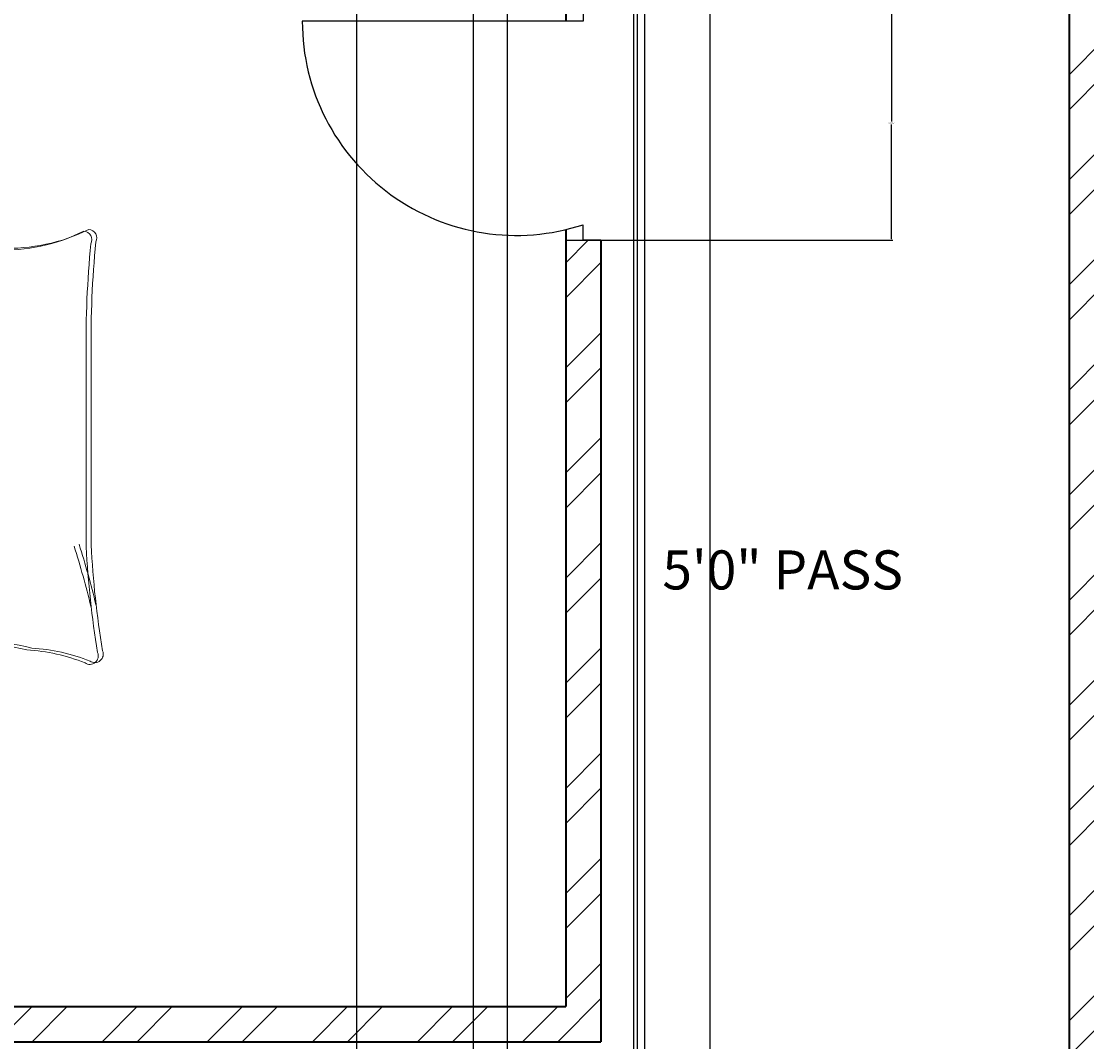
# Model space of a CAD drawing. Units: inches. Extents: x 2063 to 2617, y 1299 to 2210.
# Tile 7 of 22: x 2202 to 2338, y 1727 to 1858. Entities that reach past the tile are written whole.
import ezdxf

# ---------------------------------------------------------------- set-up
doc = ezdxf.new("R2010")
doc.units = ezdxf.units.IN
for name, color, linetype, lineweight in [('A-ANNO-DIMS', 2, 'Continuous', 18), ('A-AREA-IDEN', 7, 'Continuous', 18), ('A-DOOR', 11, 'Continuous', 25), ('A-FURN', 8, 'Continuous', 18), ('A-WALL', 7, 'Continuous', 40)]:
    doc.layers.add(name, color=color, linetype=linetype, lineweight=lineweight)
doc.layers.add('A-WALL-PATT', color=215, linetype='Continuous', lineweight=13, true_color=0xa953a0)
doc.styles.get("Standard").update_dxf_attribs({"font": 'arial.ttf'})
doc.dimstyles.get("Standard").update_dxf_attribs({"dimtxt": 0.18, "dimasz": 0.18, "dimexe": 0.18, "dimexo": 0.0625, "dimgap": 0.09, "dimtad": 0, "dimtih": 1, "dimtoh": 1, "dimdec": 4, "dimzin": 0, "dimdsep": 46, "dimtxsty": 'Standard', "dimcen": 0.09, "dimadec": 0, "dimazin": 0, "dimtfac": 1, "dimtdec": 4, "dimtofl": 0, "dimtmove": 0, "dimatfit": 3, "dimfxl": 1, "dimtolj": 1, "dimtzin": 0, "dimarcsym": 0})

# ---------------------------------------------------------------- blocks, each defined once
blk = doc.blocks.new('BED-DOUBLE')
for p, q in [((3.48, 63.33), (3.48, 81.44)), ((3.48, 63.33), (3.48, 81.44)), ((3.48, 81.44), (51.49, 81.44)), ((3.7, 62.69), (3.7, 80.8)), ((3.7, 62.69), (3.7, 80.8)), ((51.27, 81.44), (51.27, 54.83)), ((51.27, 81.44), (51.27, 54.83)), ((51.49, 81.44), (51.49, 80.8)), ((51.49, 80.8), (51.49, 54.19)), ((51.49, 80.8), (51.49, 54.19)), ((3.48, 79.91), (51.27, 79.91)), ((3.48, 79.91), (51.27, 79.91)), ((3.7, 79.27), (51.49, 79.27)), ((3.7, 79.27), (51.49, 79.27)), ((24.54, 79), (25.98, 79.57)), ((24.54, 79), (25.98, 79.57)), ((25.98, 79.57), (26.56, 74.22)), ((25.98, 79.57), (26.56, 74.22)), ((3.89, 78.13), (4.47, 74.95)), ((3.9, 78.11), (8.18, 78.43)), ((3.9, 78.11), (8.18, 78.43)), ((3.9, 78.13), (4.47, 74.95)), ((8.18, 78.43), (8.29, 78.42)), ((8.18, 78.43), (8.29, 78.42)), ((8.29, 78.42), (12.11, 78.13)), ((8.29, 78.42), (12.11, 78.13)), ((12.11, 78.13), (17.6, 77.12)), ((12.11, 78.13), (17.6, 77.12)), ((14.86, 77.69), (16.88, 78.42)), ((14.86, 77.69), (16.88, 78.42)), ((16.88, 78.42), (19.77, 79.14)), ((16.88, 78.42), (19.77, 79.14)), ((17.11, 77.78), (20, 78.5)), ((17.11, 77.78), (20, 78.5)), ((19.77, 79.14), (20.09, 79.14)), ((19.77, 79.14), (20.09, 79.14)), ((20, 78.5), (20.32, 78.5)), ((20, 78.5), (20.32, 78.5)), ((20.09, 79.14), (24.54, 79)), ((20.09, 79.14), (24.54, 79)), ((20.32, 78.5), (24.77, 78.36)), ((20.32, 78.5), (24.77, 78.36)), ((24.77, 78.36), (26.21, 78.93)), ((24.77, 78.36), (26.21, 78.93)), ((26.21, 78.93), (26.79, 73.58)), ((26.21, 78.93), (26.79, 73.58)), ((27.98, 78.95), (27.73, 73.58)), ((27.98, 78.95), (27.73, 73.58)), ((28.21, 78.31), (27.96, 72.94)), ((28.21, 78.31), (27.96, 72.94)), ((29.46, 78.46), (27.98, 78.95)), ((29.46, 78.46), (27.98, 78.95)), ((29.68, 77.83), (28.21, 78.31)), ((29.68, 77.83), (28.21, 78.31)), ((33.88, 78.89), (29.46, 78.46)), ((33.88, 78.89), (29.46, 78.46)), ((34.11, 78.25), (29.68, 77.83)), ((34.11, 78.25), (29.68, 77.83)), ((34.21, 78.91), (33.88, 78.89)), ((34.2, 78.91), (33.88, 78.89)), ((34.43, 78.27), (34.11, 78.25)), ((34.43, 78.27), (34.11, 78.25)), ((37.14, 78.37), (34.2, 78.91)), ((37.14, 78.37), (34.21, 78.91)), ((37.36, 77.73), (34.43, 78.27)), ((37.36, 77.73), (34.43, 78.27)), ((41.91, 78.37), (36.5, 77.02)), ((41.91, 78.37), (36.5, 77.02)), ((39.2, 77.77), (37.14, 78.37)), ((39.2, 77.77), (37.14, 78.37)), ((45.71, 78.9), (41.91, 78.37)), ((45.71, 78.9), (41.91, 78.37)), ((45.94, 78.26), (42.14, 77.73)), ((45.94, 78.26), (42.14, 77.73)), ((50.11, 78.89), (44.71, 78.98)), ((44.71, 78.98), (45.71, 78.9)), ((50.11, 78.89), (44.71, 78.98)), ((44.71, 78.98), (45.71, 78.9)), ((50.34, 78.25), (44.94, 78.34)), ((44.94, 78.34), (45.94, 78.26)), ((50.34, 78.25), (44.94, 78.34)), ((44.94, 78.34), (45.94, 78.26)), ((50.11, 78.89), (49.73, 75.68)), ((50.11, 78.89), (49.73, 75.68)), ((50.34, 78.25), (49.96, 75.04)), ((50.34, 78.25), (49.96, 75.04)), ((4.12, 77.49), (4.7, 74.31)), ((4.12, 77.49), (4.7, 74.31)), ((4.13, 77.47), (8.41, 77.8)), ((4.13, 77.47), (8.41, 77.8)), ((8.41, 77.8), (8.51, 77.78)), ((8.41, 77.8), (8.51, 77.78)), ((8.51, 77.78), (12.34, 77.49)), ((8.51, 77.78), (12.34, 77.49)), ((12.34, 77.49), (17.83, 76.48)), ((12.34, 77.49), (17.83, 76.48)), ((15.08, 77.05), (17.11, 77.78)), ((15.08, 77.05), (17.11, 77.78)), ((42.14, 77.73), (36.72, 76.38)), ((42.14, 77.73), (36.72, 76.38)), ((39.43, 77.13), (37.36, 77.73)), ((39.43, 77.13), (37.36, 77.73)), ((5.05, 72.49), (6.06, 75.24)), ((5.05, 72.49), (6.06, 75.24)), ((49.31, 73.19), (48.13, 75.87)), ((49.31, 73.19), (48.13, 75.87)), ((49.54, 72.55), (48.36, 75.23)), ((49.54, 72.55), (48.36, 75.23)), ((49.73, 75.68), (50.33, 73.11)), ((49.73, 75.68), (50.33, 73.11)), ((4.47, 74.95), (4.04, 72.34)), ((4.47, 74.95), (4.04, 72.34)), ((4.7, 74.31), (4.27, 71.7)), ((4.7, 74.31), (4.27, 71.7)), ((5.28, 71.85), (6.29, 74.6)), ((5.28, 71.85), (6.29, 74.6)), ((26.56, 74.22), (27.14, 71.04)), ((26.56, 74.22), (27.14, 71.04)), ((49.96, 75.04), (50.56, 72.47)), ((49.96, 75.04), (50.56, 72.47)), ((4.47, 68.87), (5.05, 72.49)), ((4.47, 68.87), (5.05, 72.49)), ((26.79, 73.58), (27.37, 70.4)), ((26.79, 73.58), (27.37, 70.4)), ((27.73, 73.58), (27.36, 70.37)), ((27.73, 73.58), (27.36, 70.37)), ((27.96, 72.94), (27.58, 69.73)), ((27.96, 72.94), (27.58, 69.73)), ((50.11, 69.61), (49.31, 73.19)), ((50.11, 69.61), (49.31, 73.19)), ((50.34, 68.98), (49.54, 72.55)), ((50.34, 68.98), (49.54, 72.55)), ((50.33, 73.11), (49.81, 72.06)), ((50.33, 73.11), (49.82, 72.06)), ((50.56, 72.47), (50.04, 71.42)), ((50.56, 72.47), (50.04, 71.42)), ((4.04, 72.34), (4.62, 71.33)), ((4.04, 72.34), (4.62, 71.33)), ((4.27, 71.7), (4.85, 70.69)), ((4.27, 71.7), (4.85, 70.69)), ((4.7, 68.23), (5.28, 71.85)), ((4.7, 68.23), (5.28, 71.85)), ((27.14, 71.04), (27.14, 69.74)), ((27.14, 71.04), (27.14, 69.74)), ((27.14, 69.74), (26.56, 67.86)), ((27.14, 69.74), (26.56, 67.86)), ((27.36, 70.37), (27.44, 69.07)), ((27.36, 70.37), (27.44, 69.07)), ((27.37, 70.4), (27.37, 69.1)), ((27.37, 70.4), (27.37, 69.1)), ((27.58, 69.73), (27.66, 68.43)), ((27.58, 69.73), (27.66, 68.43)), ((4.76, 67.28), (4.47, 68.87)), ((4.76, 67.28), (4.47, 68.87)), ((27.37, 69.1), (26.79, 67.22)), ((27.37, 69.1), (26.79, 67.22)), ((27.44, 69.07), (28.13, 67.23)), ((27.44, 69.07), (28.13, 67.23)), ((27.66, 68.43), (28.36, 66.59)), ((27.66, 68.43), (28.36, 66.59)), ((49.92, 68.01), (50.11, 69.61)), ((49.92, 68.01), (50.11, 69.61)), ((50.15, 67.37), (50.34, 68.98)), ((50.15, 67.37), (50.34, 68.98)), ((4.18, 64.1), (4.76, 67.28)), ((4.18, 64.1), (4.76, 67.28)), ((4.99, 66.64), (4.7, 68.23)), ((4.99, 66.64), (4.7, 68.23)), ((26.56, 67.86), (26.56, 65.18)), ((26.56, 67.86), (26.56, 65.18)), ((26.79, 67.22), (26.79, 64.54)), ((26.79, 67.22), (26.79, 64.54)), ((28.13, 67.23), (28.3, 64.55)), ((28.13, 67.23), (28.3, 64.55)), ((50.7, 64.87), (49.92, 68.01)), ((50.7, 64.87), (49.92, 68.01)), ((50.93, 64.23), (50.15, 67.37)), ((50.93, 64.23), (50.15, 67.37)), ((4.41, 63.46), (4.99, 66.64)), ((4.41, 63.46), (4.99, 66.64)), ((6.38, 65.82), (10.41, 65.15)), ((6.38, 65.82), (10.41, 65.15)), ((24.1, 65.18), (20.96, 66.27)), ((24.1, 65.18), (20.96, 66.27)), ((24.33, 64.54), (21.19, 65.63)), ((24.33, 64.54), (21.19, 65.63)), ((28.36, 66.59), (28.53, 63.91)), ((28.36, 66.59), (28.53, 63.91)), ((30.75, 64.7), (33.82, 65.99)), ((30.75, 64.7), (33.82, 65.99)), ((32.56, 65.82), (36.6, 65.15)), ((32.56, 65.82), (36.6, 65.15)), ((9.28, 64.83), (4.18, 64.1)), ((9.28, 64.83), (4.18, 64.1)), ((9.51, 64.19), (4.41, 63.46)), ((9.51, 64.19), (4.41, 63.46)), ((6.61, 65.18), (10.64, 64.51)), ((6.61, 65.18), (10.64, 64.51)), ((10.41, 65.15), (9.28, 64.83)), ((10.41, 65.15), (9.28, 64.83)), ((10.64, 64.51), (9.51, 64.19)), ((10.64, 64.51), (9.51, 64.19)), ((10.41, 65.15), (17.42, 64.72)), ((10.41, 65.15), (17.42, 64.72)), ((10.64, 64.51), (17.65, 64.08)), ((10.64, 64.51), (17.65, 64.08)), ((17.42, 64.72), (19.38, 65.27)), ((17.42, 64.72), (19.38, 65.27)), ((17.65, 64.08), (19.61, 64.64)), ((17.65, 64.08), (19.61, 64.64)), ((19.38, 65.27), (24.52, 64.87)), ((19.38, 65.27), (24.52, 64.87)), ((19.61, 64.64), (24.74, 64.23)), ((19.61, 64.64), (24.74, 64.23)), ((26.56, 65.18), (24.1, 65.18)), ((26.56, 65.18), (24.1, 65.18)), ((26.79, 64.54), (24.33, 64.54)), ((26.79, 64.54), (24.33, 64.54)), ((28.3, 64.55), (30.75, 64.7)), ((28.3, 64.55), (30.75, 64.7)), ((30.98, 64.06), (34.05, 65.35)), ((30.98, 64.06), (34.05, 65.35)), ((32.79, 65.18), (36.83, 64.51)), ((32.79, 65.18), (36.82, 64.51)), ((36.6, 65.15), (43.61, 64.72)), ((36.6, 65.15), (43.61, 64.72)), ((36.82, 64.51), (43.83, 64.08)), ((36.83, 64.51), (43.84, 64.08)), ((43.61, 64.72), (45.57, 65.27)), ((43.61, 64.72), (45.57, 65.27)), ((43.83, 64.08), (45.8, 64.64)), ((43.84, 64.08), (45.8, 64.64)), ((45.57, 65.27), (50.7, 64.87)), ((45.57, 65.27), (50.7, 64.87)), ((45.8, 64.64), (50.93, 64.23)), ((45.8, 64.64), (50.93, 64.23)), ((28.53, 63.91), (30.98, 64.06)), ((28.53, 63.91), (30.98, 64.06)), ((30.26, 64.06), (34.45, 57.57)), ((30.26, 64.06), (34.45, 57.57)), ((30.49, 63.42), (34.68, 56.93)), ((30.49, 63.42), (34.68, 56.93)), ((40.64, 61.13), (32.31, 64.06)), ((40.64, 61.13), (32.31, 64.06)), ((40.87, 60.49), (32.53, 63.42)), ((40.87, 60.49), (32.54, 63.42)), ((46.22, 59.11), (40.64, 61.13)), ((46.22, 59.11), (40.64, 61.13)), ((46.45, 58.48), (40.87, 60.49)), ((46.45, 58.48), (40.87, 60.49)), ((49.16, 56.95), (46.22, 59.11)), ((49.16, 56.95), (46.22, 59.11)), ((34.45, 57.57), (36.15, 53.08)), ((34.45, 57.57), (36.15, 53.08)), ((49.39, 56.31), (46.45, 58.48)), ((49.39, 56.31), (46.45, 58.48)), ((34.68, 56.93), (36.38, 52.44)), ((34.68, 56.93), (36.38, 52.44)), ((52.87, 53.7), (49.16, 56.95)), ((52.87, 53.7), (49.16, 56.95)), ((53.1, 53.06), (49.39, 56.31)), ((53.1, 53.06), (49.39, 56.31)), ((44.36, 53.08), (48.23, 53.39)), ((44.36, 53.08), (48.23, 53.39)), ((48.23, 53.39), (51.33, 53.08)), ((48.23, 53.39), (51.33, 53.08)), ((51.33, 53.08), (52.87, 53.7)), ((51.33, 53.08), (52.87, 53.7)), ((52.95, 51.95), (52.87, 53.7, 3.87)), ((52.95, 51.95), (52.87, 53.7, 3.87)), ((36.15, 53.08), (36.46, 51.07)), ((36.15, 53.08), (36.46, 51.07)), ((36.38, 52.44), (36.69, 50.43)), ((36.38, 52.44), (36.69, 50.43)), ((38.94, 51.69), (40.95, 52.61)), ((38.94, 51.69), (40.95, 52.61)), ((39.17, 51.05), (41.18, 51.97)), ((39.17, 51.05), (41.18, 51.97)), ((40.95, 52.61), (44.36, 53.08)), ((40.95, 52.61), (44.36, 53.08)), ((41.18, 51.97), (44.59, 52.44)), ((41.18, 51.97), (44.59, 52.44)), ((44.59, 52.44), (48.46, 52.75)), ((44.59, 52.44), (48.46, 52.75)), ((48.46, 52.75), (51.56, 52.44)), ((48.46, 52.75), (51.56, 52.44)), ((51.56, 52.44), (53.1, 53.06)), ((51.56, 52.44), (53.1, 53.06)), ((53.18, 51.31), (53.1, 53.06, 3.87)), ((53.18, 51.31), (53.1, 53.06, 3.87)), ((36.46, 51.07), (38.94, 51.69)), ((36.46, 51.07), (38.94, 51.69)), ((36.69, 50.43), (39.17, 51.05)), ((36.69, 50.43), (39.17, 51.05)), ((15.06, 2.2), (39.68, 2.2)), ((15.06, 2.2), (39.68, 2.2)), ((15.29, 1.56), (39.91, 1.56)), ((15.29, 1.56), (39.91, 1.56))]:
    blk.add_line(p, q)
for centre, radius, start, end in [((21.36, -100.61), 164.97, 86.0865, 96.7821), ((21.36, -100.61), 164.97, 86.0865, 96.7821), ((85.16, 61.35), 83.31, 178.7218, 185.604), ((85.16, 61.35), 83.31, 178.7218, 185.604), ((21.59, -101.25), 164.97, 86.0865, 96.7821), ((21.59, -101.25), 164.97, 86.0865, 96.7821), ((85.39, 60.71), 83.31, 178.7218, 185.604), ((85.39, 60.71), 83.31, 178.7218, 185.604), ((17.76, -74.87), 129.02, 81.7845, 96.9006), ((17.76, -74.87), 129.02, 81.7845, 96.9006), ((17.98, -75.51), 129.02, 81.7845, 96.9006), ((17.98, -75.51), 129.02, 81.7845, 96.9006), ((-167.31, 50.27), 170.11, 358.4762, 1.0082), ((-167.31, 50.27), 170.11, 358.4762, 1.0082), ((-167.08, 49.63), 170.11, 358.4762, 1.0082), ((-167.08, 49.63), 170.11, 358.4762, 1.0082), ((31.15, 79.96), 29.65, 280.6617, 289.8806), ((31.15, 79.96), 29.65, 280.6617, 289.8806), ((43.74, 46.38), 6.22, 78.6608, 113.7384), ((43.74, 46.38), 6.22, 78.6608, 113.7384), ((43.97, 45.74), 6.22, 78.6608, 113.7384), ((43.97, 45.74), 6.22, 78.6608, 113.7384), ((51.33, 88.1), 36.18, 259.8763, 272.5657), ((51.33, 88.1), 36.18, 259.8763, 272.5657), ((182.27, 45.13), 129.5, 176.9791, 183.8365), ((182.27, 45.13), 129.5, 176.9791, 183.8365), ((36.64, 51), 0.185, 160.2464, 271.1377), ((36.64, 51), 0.185, 160.2464, 271.1377), ((31.38, 79.32), 29.65, 280.6617, 289.8806), ((31.38, 79.32), 29.65, 280.6617, 289.8806), ((51.56, 87.46), 36.18, 259.8763, 272.5657), ((51.56, 87.46), 36.18, 259.8763, 272.5657), ((182.49, 44.49), 129.5, 176.9791, 183.8365), ((182.49, 44.49), 129.5, 176.9791, 183.8365), ((36.87, 50.36), 0.185, 160.2464, 271.1377), ((36.86, 50.36), 0.185, 160.2464, 271.1377), ((484.82, 30.83), 482.31, 178.2277, 181.7185), ((484.82, 30.83), 482.31, 178.2277, 181.7185), ((485.05, 30.19), 482.31, 178.2277, 181.7185), ((485.05, 30.19), 482.31, 178.2277, 181.7185), ((-4508.74, 13.62), 4561.86, 0.00217, 0.28689), ((-4508.74, 13.62), 4561.86, 0.00217, 0.28689), ((-4508.51, 12.98), 4561.86, 0.00217, 0.28689), ((-4508.51, 12.98), 4561.86, 0.00217, 0.28689), ((-26.9, 16.93), 29.63, 346.0648, 358.9113), ((-26.9, 16.93), 29.63, 346.0648, 358.9113), ((-26.67, 16.29), 29.63, 346.0648, 358.9113), ((-26.67, 16.29), 29.63, 346.0648, 358.9113), ((76.16, 12.78), 23.07, 177.4714, 206.4681), ((76.16, 12.78), 23.07, 177.4714, 206.4681), ((76.39, 12.14), 23.07, 177.4714, 206.4681), ((76.39, 12.14), 23.07, 177.4714, 206.4681), ((-21.66, 11.17), 23.56, 337.9751, 356.652), ((-21.66, 11.17), 23.56, 337.9751, 356.652), ((-21.43, 10.53), 23.56, 337.9751, 356.652), ((-21.43, 10.53), 23.56, 337.9751, 356.652), ((-17.22, 105.16), 106.46, 283.3832, 287.7053), ((-17.22, 105.16), 106.46, 283.3832, 287.7053), ((-16.99, 104.52), 106.46, 283.3832, 287.7053), ((-16.99, 104.52), 106.46, 283.3832, 287.7053), ((1.09, 1.73), 1.09, 146.1736, 293.4781), ((1.09, 1.73), 1.09, 146.1736, 293.4781), ((1.32, 1.09), 1.09, 146.1736, 293.4781), ((1.32, 1.09), 1.09, 146.1736, 293.4781), ((21.43, -119.39), 121.76, 92.9958, 99.4091), ((21.43, -119.39), 121.76, 92.9958, 99.4091), ((21.66, -120.03), 121.76, 92.9958, 99.4091), ((21.66, -120.03), 121.76, 92.9958, 99.4091), ((41.15, -130.83), 133.04, 84.4998, 90.6351), ((41.15, -130.83), 133.04, 84.4998, 90.6351), ((41.38, -131.47), 133.04, 84.4998, 90.6351), ((41.38, -131.47), 133.04, 84.4998, 90.6351), ((54.41, 2.57), 1.1, 242.6588, 356.02), ((54.41, 2.57), 1.1, 242.6588, 356.02), ((54.64, 1.93), 1.1, 242.6588, 356.02), ((54.64, 1.93), 1.1, 242.6588, 356.02)]:
    blk.add_arc(centre, radius, start, end)
blk = doc.blocks.new('*D50')
at = {"layer": 'A-ANNO-DIMS', "color": 0, "lineweight": -2, "transparency": 16777216}
for p, q in [((2264.14, 2124.25), (2264.14, 1317.7)), ((2280.35, 2124.25), (2280.35, 1317.7)), ((2264.32, 1317.88), (2271.79, 1317.88)), ((2280.17, 1317.88), (2272.7, 1317.88))]:
    blk.add_line(p, q, dxfattribs=at)
at = {"layer": 'A-ANNO-DIMS', "color": 0, "transparency": 16777216}
for points in [[(2264.32, 1317.91), (2264.32, 1317.85), (2264.14, 1317.88)], [(2280.17, 1317.91), (2280.17, 1317.85), (2280.35, 1317.88)]]:
    blk.add_solid(points, dxfattribs=at)
at = {"layer": 'Defpoints', "color": 0, "transparency": 16777216}
for p in [(2264.14, 2124.31), (2280.35, 2124.31), (2280.35, 1317.88)]:
    blk.add_point(p, dxfattribs=at)
at = {"layer": 'A-ANNO-DIMS', "color": 0, "transparency": 16777216, "insert": (2272.25, 1317.88), "char_height": 0.18, "attachment_point": 5}
blk.add_mtext('\\A1;16.204', dxfattribs=at)
blk = doc.blocks.new('*D59')
at = {"layer": 'A-ANNO-DIMS', "color": 0, "lineweight": -2, "transparency": 16777216}
for p, q in [((2290.14, 1554.56), (2290.14, 2170.74)), ((2290.32, 2170.56), (2315.07, 2170.56)), ((2340.46, 2170.56), (2315.72, 2170.56)), ((2340.64, 1554.56), (2340.64, 2170.74))]:
    blk.add_line(p, q, dxfattribs=at)
at = {"layer": 'A-ANNO-DIMS', "color": 0, "transparency": 16777216}
for points in [[(2290.32, 2170.59), (2290.32, 2170.53), (2290.14, 2170.56)], [(2340.46, 2170.59), (2340.46, 2170.53), (2340.64, 2170.56)]]:
    blk.add_solid(points, dxfattribs=at)
at = {"layer": 'Defpoints', "color": 0, "transparency": 16777216}
for p in [(2340.64, 2170.56), (2290.14, 1554.5), (2340.64, 1554.5)]:
    blk.add_point(p, dxfattribs=at)
at = {"layer": 'A-ANNO-DIMS', "color": 0, "transparency": 16777216, "insert": (2315.39, 2170.56), "char_height": 0.18, "attachment_point": 5}
blk.add_mtext('\\A1;50.5', dxfattribs=at)
blk = doc.blocks.new('*D62')
at = {"layer": 'A-ANNO-DIMS', "color": 0, "lineweight": -2, "transparency": 16777216}
for p, q in [((2259.81, 1437.87), (2259.81, 2170.74)), ((2259.99, 2170.56), (2270.4, 2170.56)), ((2281.61, 2170.56), (2271.19, 2170.56)), ((2281.79, 1437.87), (2281.79, 2170.74))]:
    blk.add_line(p, q, dxfattribs=at)
at = {"layer": 'A-ANNO-DIMS', "color": 0, "transparency": 16777216}
for points in [[(2259.99, 2170.59), (2259.99, 2170.53), (2259.81, 2170.56)], [(2281.61, 2170.59), (2281.61, 2170.53), (2281.79, 2170.56)]]:
    blk.add_solid(points, dxfattribs=at)
at = {"layer": 'Defpoints', "color": 0, "transparency": 16777216}
for p in [(2281.79, 2170.56), (2259.81, 1437.81), (2281.79, 1437.81)]:
    blk.add_point(p, dxfattribs=at)
at = {"layer": 'A-ANNO-DIMS', "color": 0, "transparency": 16777216, "insert": (2270.8, 2170.56), "char_height": 0.18, "attachment_point": 5}
blk.add_mtext('\\A1;21.98', dxfattribs=at)
blk = doc.blocks.new('*D63')
at = {"layer": 'A-ANNO-DIMS', "color": 0, "lineweight": -2, "transparency": 16777216}
for p, q in [((2244.87, 1562.37), (2244.87, 2170.74)), ((2245.05, 2170.56), (2262.4, 2170.56)), ((2280.68, 2170.56), (2263.33, 2170.56)), ((2280.86, 1562.37), (2280.86, 2170.74))]:
    blk.add_line(p, q, dxfattribs=at)
at = {"layer": 'A-ANNO-DIMS', "color": 0, "transparency": 16777216}
for points in [[(2245.05, 2170.59), (2245.05, 2170.53), (2244.87, 2170.56)], [(2280.68, 2170.59), (2280.68, 2170.53), (2280.86, 2170.56)]]:
    blk.add_solid(points, dxfattribs=at)
at = {"layer": 'Defpoints', "color": 0, "transparency": 16777216}
for p in [(2280.86, 2170.56), (2244.87, 1562.31), (2280.86, 1562.31)]:
    blk.add_point(p, dxfattribs=at)
at = {"layer": 'A-ANNO-DIMS', "color": 0, "transparency": 16777216, "insert": (2262.86, 2170.56), "char_height": 0.18, "attachment_point": 5}
blk.add_mtext('\\A1;35.995', dxfattribs=at)
blk = doc.blocks.new('*D69')
at = {"layer": 'A-ANNO-DIMS', "color": 0, "lineweight": -2, "transparency": 16777216}
for p, q in [((2271.71, 1860.05), (2313.57, 1860.05)), ((2313.39, 1859.87), (2313.39, 1845.2)), ((2313.39, 1830.17), (2313.39, 1844.84)), ((2271.71, 1829.99), (2313.57, 1829.99))]:
    blk.add_line(p, q, dxfattribs=at)
at = {"layer": 'A-ANNO-DIMS', "color": 0, "transparency": 16777216}
for points in [[(2313.36, 1859.87), (2313.42, 1859.87), (2313.39, 1860.05)], [(2313.36, 1830.17), (2313.42, 1830.17), (2313.39, 1829.99)]]:
    blk.add_solid(points, dxfattribs=at)
at = {"layer": 'Defpoints', "color": 0, "transparency": 16777216}
for p in [(2271.64, 1860.05), (2271.64, 1829.99), (2313.39, 1829.99)]:
    blk.add_point(p, dxfattribs=at)
at = {"layer": 'A-ANNO-DIMS', "color": 0, "transparency": 16777216, "insert": (2313.39, 1845.02), "char_height": 0.18, "attachment_point": 5}
blk.add_mtext('\\A1;30.057', dxfattribs=at)

msp = doc.modelspace()

# ---------------------------------------------------------------- hatches: boundary and pattern name
at = {"layer": 'A-WALL-PATT'}
h = msp.add_hatch(dxfattribs=at)
h.set_pattern_fill('ANSI32', color=256)
h.paths.add_polyline_path([(2553.6442, 2128.8122), (2511.1703, 2128.8122), (2511.1703, 2124.3122), (2549.1442, 2124.3122), (2549.1442, 2095.662), (2553.6442, 2095.662)])
h.paths.add_polyline_path([(2553.6442, 2035.662), (2549.1442, 2035.662), (2549.1442, 1980.3122), (2503.7214, 1980.3122), (2503.7214, 1975.8122), (2549.1442, 1975.8122), (2549.1442, 1962.9693), (2553.6442, 1962.9693)])
h.paths.add_polyline_path([(2553.6442, 1938.9693), (2549.1442, 1938.9693), (2549.1442, 1927.8122), (2477.1442, 1927.8122), (2477.1442, 1975.8122), (2481.2918, 1975.8122), (2481.2918, 1980.3122), (2453.2648, 1980.3122), (2453.2648, 1975.8122), (2472.6442, 1975.8122), (2472.6442, 1868.3122), (2400.6442, 1868.3122), (2400.6442, 1861.3782), (2405.1442, 1861.3782), (2405.1442, 1863.8122), (2480.9699, 1863.8122), (2480.9699, 1866.0622), (2480.9699, 1868.3122), (2477.1442, 1868.3122), (2477.1442, 1923.3122), (2549.1442, 1923.3122), (2549.1442, 1908.8504), (2553.6442, 1908.8504)])
h.paths.add_polyline_path([(2553.6442, 1884.8504), (2549.1442, 1884.8504), (2549.1442, 1868.3122), (2501.0636, 1868.3122), (2501.0636, 1863.8122), (2549.1442, 1863.8122), (2549.1442, 1826.0298), (2553.6442, 1826.0298)])
h.paths.add_polyline_path([(2388.1504, 1980.3122), (2340.6442, 1980.3122), (2340.6442, 2124.3122), (2358.7501, 2124.3122), (2358.7501, 2128.8122), (2316.3482, 2128.8122), (2316.3482, 2124.3122), (2336.1442, 2124.3122), (2336.1442, 1980.3122), (2289.1737, 1980.3122), (2289.1737, 1975.8122), (2336.1442, 1975.8122), (2336.1442, 1619.3122), (2333.1433, 1619.3122), (2333.1433, 1614.8122), (2344.1671, 1614.8122), (2344.1671, 1617.0622), (2344.1671, 1619.3122), (2340.6442, 1619.3122), (2340.6442, 1975.8122), (2388.1504, 1975.8122), (2388.1504, 1978.0622)])
h.paths.add_polyline_path([(2290.1442, 1614.8122), (2301.4594, 1614.8122), (2301.4594, 1617.0622), (2301.4594, 1619.3122), (2285.6442, 1619.3122), (2285.6442, 1566.8122), (2280.8619, 1566.8122), (2280.8619, 1564.5622), (2280.8619, 1562.3122), (2285.6442, 1562.3122), (2285.6442, 1442.3122), (2281.7879, 1442.3122), (2281.7879, 1437.8122), (2285.6442, 1437.8122), (2285.6442, 1401.8122), (2290.1442, 1401.8122)])
h.paths.add_polyline_path([(2549.1442, 1731.8122), (2405.1442, 1731.8122), (2405.1442, 1834.4638), (2402.8942, 1834.4638), (2400.6442, 1834.4638), (2400.6442, 1727.3122), (2549.1442, 1727.3122)])
h.paths.add_polyline_path([(2553.6442, 1766.0298), (2551.3942, 1766.0298), (2549.1442, 1766.0298), (2549.1442, 1686.7767), (2553.6442, 1686.7767)])
h.paths.add_polyline_path([(2553.6442, 1638.7767), (2551.3942, 1638.7767), (2549.1442, 1638.7767), (2549.1442, 1619.3122), (2448.6442, 1619.3122), (2448.6442, 1610.5671), (2450.8942, 1610.5671), (2453.1442, 1610.5671), (2453.1442, 1614.8122), (2549.1442, 1614.8122), (2549.1442, 1601.6421), (2553.6442, 1601.6421)])
h.paths.add_polyline_path([(2553.6442, 1577.6421), (2551.3942, 1577.6421), (2549.1442, 1577.6421), (2549.1442, 1566.8122), (2453.1442, 1566.8122), (2453.1442, 1591.5045), (2451.0335, 1591.5045), (2448.6442, 1591.5045), (2448.6442, 1566.8122), (2434.0475, 1566.8122), (2434.0475, 1562.3122), (2549.1442, 1562.3122), (2549.1442, 1533.48), (2553.6442, 1533.48)])
h.paths.add_polyline_path([(2553.6442, 1473.48), (2549.1442, 1473.48), (2549.1442, 1442.3122), (2502.6258, 1442.3122), (2502.6258, 1437.8122), (2549.1442, 1437.8122), (2549.1442, 1401.8122), (2553.6442, 1401.8122)])
h.paths.add_polyline_path([(2395.6442, 1562.3122), (2400.0901, 1562.3122), (2400.0901, 1564.5622), (2400.0901, 1566.8122), (2395.6442, 1566.8122), (2395.6442, 1619.3122), (2379.1127, 1619.3122), (2379.1127, 1614.8122), (2391.1442, 1614.8122), (2391.1442, 1401.8122), (2395.6442, 1401.8122), (2395.6442, 1437.8122), (2399.2425, 1437.8122), (2399.2425, 1440.0622), (2399.2425, 1442.3122), (2395.6442, 1442.3122)])
h.paths.add_polyline_path([(2442.6258, 1442.3122), (2419.6262, 1442.3122), (2419.6262, 1437.8122), (2442.6258, 1437.8122), (2442.6258, 1440.0622)])
h.paths.add_polyline_path([(2127.6442, 1480.2532), (2125.3942, 1480.2532), (2123.1442, 1480.2532), (2123.1442, 1401.8122), (2127.6442, 1401.8122), (2127.6442, 1437.8122), (2145.1538, 1437.8122), (2145.1538, 1440.0622), (2145.1538, 1442.3122), (2127.6442, 1442.3122)])
h.paths.add_polyline_path([(2259.809, 1442.3122), (2205.1538, 1442.3122), (2205.1538, 1437.8122), (2259.809, 1437.8122), (2259.809, 1440.0622)])
h.paths.add_polyline_path([(2127.6442, 1659.7652), (2123.1442, 1659.7652), (2123.1442, 1605.5161), (2125.3942, 1605.5161), (2127.6442, 1605.5161), (2127.6442, 1614.8122), (2223.6442, 1614.8122), (2223.6442, 1611.2723), (2228.1442, 1611.2723), (2228.1442, 1619.3122), (2127.6442, 1619.3122)])
h.paths.add_polyline_path([(2244.8673, 1566.8122), (2228.1442, 1566.8122), (2228.1442, 1590.8122), (2225.8942, 1590.8122), (2223.6442, 1590.8122), (2223.6442, 1566.8122), (2127.6442, 1566.8122), (2127.6442, 1581.5161), (2123.1442, 1581.5161), (2123.1442, 1540.2532), (2127.6442, 1540.2532), (2127.6442, 1562.3122), (2244.8673, 1562.3122), (2244.8673, 1564.5622)])
h.paths.add_polyline_path([(2172.5174, 1868.3122), (2127.6442, 1868.3122), (2127.6442, 1886.5833), (2123.1442, 1886.5833), (2123.1442, 1832.6633), (2127.6442, 1832.6633), (2127.6442, 1863.8122), (2172.5174, 1863.8122), (2172.5174, 1866.0622)])
h.paths.add_polyline_path([(2276.1442, 1868.3122), (2204.1442, 1868.3122), (2204.1442, 1923.3122), (2204.1442, 1975.8122), (2224.8362, 1975.8122), (2224.8362, 1978.1097), (2224.8362, 1980.3122), (2195.0729, 1980.3122), (2195.0729, 1978.0622), (2195.0729, 1975.8122), (2199.6442, 1975.8122), (2199.6442, 1927.8122), (2127.6442, 1927.8122), (2127.6442, 1942.3492), (2123.1442, 1942.3492), (2123.1442, 1910.5833), (2127.6442, 1910.5833), (2127.6442, 1923.3122), (2199.6442, 1923.3122), (2199.6442, 1868.3122), (2194.8228, 1868.3122), (2194.8228, 1864.7337), (2194.8228, 1863.8122), (2271.6442, 1863.8122), (2271.6442, 1860.0507), (2276.1442, 1860.0507)])
h.paths.add_polyline_path([(2276.1442, 1829.994), (2273.8942, 1829.994), (2271.6442, 1829.994), (2271.6442, 1731.8122), (2127.6442, 1731.8122), (2127.6442, 1772.6633), (2123.1442, 1772.6633), (2123.1442, 1707.7652), (2127.6442, 1707.7652), (2127.6442, 1727.3122), (2276.1442, 1727.3122)])
h.paths.add_polyline_path([(2127.6442, 2022.1152), (2123.1442, 2022.1152), (2123.1442, 1966.3492), (2127.6442, 1966.3492), (2127.6442, 1975.8122), (2174.2082, 1975.8122), (2174.2082, 1978.0622), (2174.2082, 1980.3122), (2127.6442, 1980.3122)])
h.paths.add_polyline_path([(2361.9755, 1678.588), (2398.4558, 1678.588), (2398.4558, 1697.2453), (2361.9755, 1697.2453)], flags=9)
h.paths.add_polyline_path([(2351.5397, 1780.4072), (2386.1987, 1780.4072), (2386.1987, 1790.7107), (2351.5397, 1790.7107)], flags=25)
h.paths.add_polyline_path([(2350.6753, 1940.9321), (2387.6024, 1940.9321), (2387.6024, 1959.5894), (2350.6753, 1959.5894)], flags=25)
h.paths.add_polyline_path([(2254.9545, 1684.638), (2295.0943, 1684.638), (2295.0943, 1703.2953), (2254.9545, 1703.2953)], flags=9)
h.paths.add_polyline_path([(2282.4946, 1782.4438), (2317.1535, 1782.4438), (2317.1535, 1792.7474), (2282.4946, 1792.7474)], flags=9)
h.paths.add_polyline_path([(2270.327, 1939.2854), (2307.254, 1939.2854), (2307.254, 1957.9428), (2270.327, 1957.9428)], flags=9)

# ---------------------------------------------------------------- linework, layer by layer
at = {"layer": 'A-DOOR'}
for p, q in [((2273.8942, 1860.0507), (2273.8942, 1858.0507)), ((2273.8942, 1858.0507), (2237.8942, 1858.0507)), ((2273.8942, 1829.994), (2273.8942, 1831.994)), ((2271.6442, 1829.994), (2276.1442, 1829.994)), ((2276.1442, 1829.994), (2273.8942, 1829.994))]:
    msp.add_line(p, q, dxfattribs=at)
msp.add_arc((2265.3241, 1858.0507), 27.4298, 180, 288.206324, dxfattribs=at)
at = {"layer": 'A-WALL'}
for p, q in [((2336.1442, 1975.8122), (2336.1442, 1619.3122)), ((2271.6442, 1863.8122), (2271.6442, 1858.0507)), ((2271.6442, 1831.3589), (2271.6442, 1731.8122)), ((2276.1442, 1829.994), (2276.1442, 1727.3122)), ((2127.6442, 1731.8122), (2271.6442, 1731.8122)), ((2127.6442, 1727.3122), (2276.1442, 1727.3122))]:
    msp.add_line(p, q, dxfattribs=at)

# ---------------------------------------------------------------- block references
at = {"layer": 'A-FURN', "rotation": 90}
msp.add_blockref('BED-DOUBLE', (2212.399, 1775.6548), dxfattribs=at)

# ---------------------------------------------------------------- texts
at = {"layer": 'A-AREA-IDEN', "insert": (2284.0345, 1790.2593), "char_height": 5, "attachment_point": 1}
msp.add_mtext_dynamic_manual_height_columns('5\'0" PASS', width=87.834442, gutter_width=12.5, heights=[0], dxfattribs=at)

# ---------------------------------------------------------------- dimensions: what is measured, and where the dimension line sits
at = {"layer": 'A-ANNO-DIMS'}
for base, p1, p2, override, picture, middle in [((2280.8619, 2170.5622), (2244.8673, 1562.3122), (2280.8619, 1562.3122), {"dimdec": 3, "dimlfac": 1, "dimrnd": 0, "dimzin": 0, "dimdsep": 46, "dimlunit": 2}, '*D63', (2262.8646, 2170.5622)), ((2281.7879, 2170.5622), (2259.809, 1437.8122), (2281.7879, 1437.8122), {"dimdec": 2, "dimlfac": 1, "dimrnd": 0, "dimzin": 0, "dimdsep": 46, "dimlunit": 2}, '*D62', (2270.7984, 2170.5622)), ((2340.6442, 2170.5622), (2290.1442, 1554.4994), (2340.6442, 1554.4994), {"dimdec": 1, "dimlfac": 1, "dimrnd": 0, "dimzin": 0, "dimdsep": 46, "dimlunit": 2}, '*D59', (2315.3942, 2170.5622)), ((2280.3482, 1317.8821), (2264.1442, 2124.3122), (2280.3482, 2124.3122), {"dimdec": 3, "dimlfac": 1, "dimrnd": 0, "dimzin": 0, "dimdsep": 46, "dimlunit": 2}, '*D50', (2272.2462, 1317.8821))]:
    dim = msp.add_linear_dim(base=base, p1=p1, p2=p2, dimstyle='Standard', override=override, dxfattribs=at)
    dim.commit()
    dim.dimension.update_dxf_attribs({"geometry": picture, "text_midpoint": middle})
dim = msp.add_linear_dim(base=(2313.3943, 1829.994), p1=(2271.6442, 1860.0507), p2=(2271.6442, 1829.994), angle=270, dimstyle='Standard', override={"dimdec": 3, "dimlfac": 1, "dimrnd": 0, "dimzin": 0, "dimdsep": 46, "dimlunit": 2}, dxfattribs=at)
dim.commit()
dim.dimension.update_dxf_attribs({"geometry": '*D69', "text_midpoint": (2313.3943, 1845.0224)})

doc.saveas('drawing.dxf')
